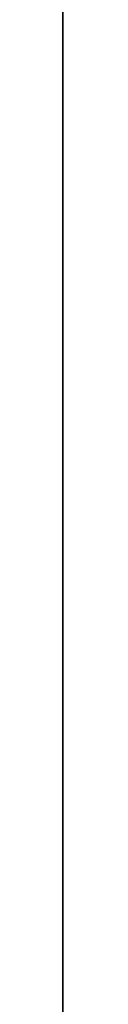
# Model space of a CAD drawing. Units: inches. Extents: x 2083 to 3317, y 1141 to 2115.
# Tile 33 of 256: x 2235.95977 to 2235.95984, y 1477.77958 to 1477.8005. Entities that reach past the tile are written whole.
import ezdxf

# ---------------------------------------------------------------- set-up
doc = ezdxf.new("R2010")
doc.units = ezdxf.units.IN
doc.layers.add('A-ANNO-DIMS', color=2, linetype='Continuous', lineweight=18)
doc.layers.add('A-WALL', color=7, linetype='Continuous', lineweight=35)
doc.layers.add('A-WALL-PATT', color=251, linetype='Continuous', lineweight=13, true_color=0x636466)
doc.styles.get("Standard").update_dxf_attribs({"font": 'arial.ttf'})
doc.dimstyles.new('ISO-25', dxfattribs={"dimtxt": 12, "dimasz": 12, "dimexe": 1.25, "dimexo": 0.625, "dimtad": 1, "dimlunit": 3, "dimtxsty": 'Standard', "dimcen": 2.5, "dimadec": 0, "dimazin": 0, "dimtfac": 1, "dimtmove": 0, "dimatfit": 3, "dimfxl": 1, "dimarcsym": 0})

# ---------------------------------------------------------------- blocks, each defined once
blk = doc.blocks.new('*D30')
at = {"layer": 'A-ANNO-DIMS', "color": 0, "lineweight": -2, "transparency": 16777216}
for p, q in [((2240.017856, 1445.273807), (2240.017856, 1448.045528)), ((2254.329327, 1445.273807), (2254.329327, 1448.045528)), ((2228.017856, 1446.795528), (2216.017856, 1446.795528)), ((2240.017856, 1446.795528), (2254.329327, 1446.795528)), ((2266.329327, 1446.795528), (2413.764866, 1446.795528))]:
    blk.add_line(p, q, dxfattribs=at)
at = {"layer": 'A-ANNO-DIMS', "color": 0, "transparency": 16777216}
for points in [[(2228.017856, 1448.795528), (2228.017856, 1444.795528), (2240.017856, 1446.795528)], [(2266.329327, 1448.795528), (2266.329327, 1444.795528), (2254.329327, 1446.795528)]]:
    blk.add_solid(points, dxfattribs=at)
at = {"layer": 'Defpoints', "color": 0, "transparency": 16777216}
for p in [(2254.329327, 1446.795528), (2240.017856, 1444.648807), (2254.329327, 1444.648807)]:
    blk.add_point(p, dxfattribs=at)
at = {"layer": 'A-ANNO-DIMS', "color": 0, "transparency": 16777216, "insert": (2346.047096, 1453.625167), "char_height": 12, "attachment_point": 5}
blk.add_mtext('WC 1\'-2 1/2" TYP.', dxfattribs=at)
blk = doc.blocks.new('*D31')
at = {"layer": 'A-ANNO-DIMS', "color": 0, "lineweight": -2, "transparency": 16777216}
for p, q in [((2237.871136, 1456.648807), (2237.871136, 1541.915179)), ((2239.392856, 1444.648807), (2236.621136, 1444.648807)), ((2237.871136, 1431.547542), (2237.871136, 1444.648807)), ((2239.392856, 1431.547542), (2236.621136, 1431.547542)), ((2237.871136, 1419.547542), (2237.871136, 1407.547542))]:
    blk.add_line(p, q, dxfattribs=at)
at = {"layer": 'A-ANNO-DIMS', "color": 0, "transparency": 16777216}
for points in [[(2235.871136, 1456.648807), (2239.871136, 1456.648807), (2237.871136, 1444.648807)], [(2235.871136, 1419.547542), (2239.871136, 1419.547542), (2237.871136, 1431.547542)]]:
    blk.add_solid(points, dxfattribs=at)
at = {"layer": 'Defpoints', "color": 0, "transparency": 16777216}
for p in [(2237.871136, 1444.648807), (2240.017856, 1444.648807), (2240.017856, 1431.547542)]:
    blk.add_point(p, dxfattribs=at)
at = {"layer": 'A-ANNO-DIMS', "color": 0, "transparency": 16777216, "insert": (2231.217486, 1505.281993), "char_height": 12, "attachment_point": 5, "rotation": 90}
blk.add_mtext('1\'-1" TYP.', dxfattribs=at)
blk = doc.blocks.new('*D45')
at = {"layer": 'A-ANNO-DIMS', "color": 0, "lineweight": -2, "transparency": 16777216}
for p, q in [((2235.959783, 1478.38636), (2235.959783, 1531.36136)), ((2418.959783, 1478.38636), (2418.959783, 1531.36136)), ((2247.959783, 1530.11136), (2406.959783, 1530.11136))]:
    blk.add_line(p, q, dxfattribs=at)
at = {"layer": 'A-ANNO-DIMS', "color": 0, "transparency": 16777216}
for points in [[(2247.959783, 1532.11136), (2247.959783, 1528.11136), (2235.959783, 1530.11136)], [(2406.959783, 1532.11136), (2406.959783, 1528.11136), (2418.959783, 1530.11136)]]:
    blk.add_solid(points, dxfattribs=at)
at = {"layer": 'Defpoints', "color": 0, "transparency": 16777216}
for p in [(2418.959783, 1530.11136), (2235.959783, 1477.76136), (2418.959783, 1477.76136)]:
    blk.add_point(p, dxfattribs=at)
at = {"layer": 'A-ANNO-DIMS', "color": 0, "transparency": 16777216, "insert": (2327.459783, 1536.867329), "char_height": 12, "attachment_point": 5}
blk.add_mtext('15\'-3"', dxfattribs=at)
blk = doc.blocks.new('*D62')
at = {"layer": 'A-ANNO-DIMS', "color": 0, "lineweight": -2, "transparency": 16777216}
for p, q in [((2235.959783, 1469.38636), (2235.959783, 1522.36136)), ((2379.959783, 1469.38636), (2379.959783, 1522.36136)), ((2247.959783, 1521.11136), (2367.959783, 1521.11136))]:
    blk.add_line(p, q, dxfattribs=at)
at = {"layer": 'A-ANNO-DIMS', "color": 0, "transparency": 16777216}
for points in [[(2247.959783, 1523.11136), (2247.959783, 1519.11136), (2235.959783, 1521.11136)], [(2367.959783, 1523.11136), (2367.959783, 1519.11136), (2379.959783, 1521.11136)]]:
    blk.add_solid(points, dxfattribs=at)
at = {"layer": 'Defpoints', "color": 0, "transparency": 16777216}
for p in [(2379.959783, 1521.11136), (2235.959783, 1468.76136), (2379.959783, 1468.76136)]:
    blk.add_point(p, dxfattribs=at)
at = {"layer": 'A-ANNO-DIMS', "color": 0, "transparency": 16777216, "insert": (2307.959783, 1527.863236), "char_height": 12, "attachment_point": 5}
blk.add_mtext('12\'-0"', dxfattribs=at)

msp = doc.modelspace()

# ---------------------------------------------------------------- hatches: boundary and pattern name
at = {"layer": 'A-WALL-PATT'}
h = msp.add_hatch(color=256, dxfattribs=at)
h.dxf.hatch_style = 1
h.paths.add_polyline_path([(3126.959783, 2020.76136), (2748.959783, 2020.76136), (2604.959783, 2020.76136), (2226.959783, 2020.76136), (2226.959783, 1702.76136), (2466.959783, 1702.76136), (2466.959783, 1582.76136), (2418.959783, 1582.76136), (2418.959783, 1477.76136), (2226.959783, 1477.76136), (2226.959783, 1263.26136), (2544.959783, 1263.26136), (2544.959783, 1411.76136), (2604.959783, 1411.76136), (2685.959783, 1411.76136), (2685.959783, 1420.76136), (2604.959783, 1420.76136), (2604.959783, 1573.76136), (2604.959783, 1702.76136), (2604.959783, 2011.76136), (2748.959783, 2011.76136), (2748.959783, 1702.76136), (2862.959783, 1702.76136), (2862.959783, 1621.76136), (2871.959783, 1621.76136), (2871.959783, 1702.76136), (2883.959783, 1702.76136), (2883.959783, 1706.939459, -0.026459), (2883.959783, 1711.76136), (2757.959783, 1711.76136), (2757.959783, 1807.76136), (2787.959783, 1807.76136), (2787.959783, 1812.26136), (2757.959783, 1812.26136), (2757.959783, 2011.76136), (2877.959783, 2011.76136), (2877.959783, 1812.26136), (2847.959783, 1812.26136), (2847.959783, 1807.76136), (2889.835742, 1807.76136), (2889.835742, 1812.26136), (2882.459783, 1812.26136), (2882.459783, 2011.76136), (3117.959783, 2011.76136), (3117.959783, 1812.26136), (2937.835742, 1812.26136), (2937.835742, 1807.76136), (2995.709783, 1807.76136), (2995.709783, 1796.117666), (3000.209783, 1796.117666), (3000.209783, 1807.76136), (3117.959783, 1807.76136), (3117.959783, 1711.76136), (3000.209783, 1711.76136), (3000.209783, 1760.117666), (2998.572705, 1760.117666, -0.020711), (2995.709783, 1760.117666), (2995.709783, 1711.76136), (2931.959783, 1711.76136), (2931.959783, 1702.76136), (3126.959783, 1702.76136)])
h.paths.add_polyline_path([(2471.459783, 2011.76136), (2471.459783, 1810.01136), (2462.716936, 1810.01136), (2462.716936, 1805.51136), (2505.959783, 1805.51136), (2505.959783, 1810.01136), (2475.959783, 1810.01136), (2475.959783, 2011.76136), (2595.959783, 2011.76136), (2595.959783, 1810.01136), (2565.959783, 1810.01136), (2565.959783, 1805.51136), (2595.959783, 1805.51136), (2595.959783, 1711.76136), (2235.959783, 1711.76136), (2235.959783, 1805.51136), (2353.709783, 1805.51136), (2353.709783, 1796.054162), (2358.209783, 1796.054162), (2358.209783, 1805.51136), (2414.716936, 1805.51136), (2414.716936, 1810.01136), (2235.959783, 1810.01136), (2235.959783, 2011.76136)], flags=16)
h.paths.add_polyline_path([(2270.204734, 1994.610008), (2270.204734, 1970.610008), (2246.204734, 1970.610008), (2246.204734, 1994.610008)], flags=0)
edge = h.paths.add_edge_path(flags=0)
edge.add_ellipse((2332.027391, 1899.798176), major_axis=(-3.042994, 3.042994), ratio=0.16825245, start_angle=-161.332166, end_angle=-156.307114, ccw=False)
edge.add_ellipse((2333.082037, 1898.74353), major_axis=(-1.054646, 1.054646), ratio=0.4535321, start_angle=-123.371019, end_angle=-94.159107)
edge = h.paths.add_edge_path(flags=0)
edge.add_ellipse((2332.027391, 1968.87629), major_axis=(3.042994, 3.042994), ratio=0.16825245, start_angle=18.667834, end_angle=23.692886)
edge.add_spline(control_points=[(2332.925596, 1970.691105), (2332.226768, 1970.3361), (2330.893709, 1969.658905), (2328.41308, 1970.932138), (2327.203934, 1967.748712), (2324.709596, 1969.955589), (2322.532822, 1967.012354), (2320.012846, 1971.295812), (2317.680308, 1968.157845), (2316.040526, 1967.102047), (2315.426904, 1966.809602)], knot_values=[0, 0, 0, 0, 2.267059, 4.324559, 6.685584, 8.878641, 11.121502, 14.300359, 17.755284, 19.732645, 19.732645, 19.732645, 19.732645], degree=3, periodic=0)
edge.add_ellipse((2332.027391, 1968.87629), major_axis=(3.042994, 3.042994), ratio=0.16825245, start_angle=18.667834, end_angle=23.692886, ccw=False)
edge.add_ellipse((2333.082037, 1969.930936), major_axis=(1.054646, 1.054646), ratio=0.4535321, start_angle=56.628981, end_angle=85.840893, ccw=False)
edge = h.paths.add_edge_path(flags=0)
edge.add_spline(control_points=[(2296.428287, 1967.987908), (2293.627804, 1965.336314), (2287.703624, 1959.727094), (2299.74386, 1949.995699), (2294.532591, 1935.668528), (2290.573228, 1920.603512), (2293.394124, 1909.973691), (2296.185407, 1904.966543)], knot_values=[0.099185, 0.099185, 0.099185, 0.099185, 0.345301, 0.619822, 0.982653, 1.386093, 1.810555, 1.810555, 1.810555, 1.810555], degree=3, periodic=0)
edge.add_spline(control_points=[(2296.185407, 1904.966543), (2297.383582, 1902.6193), (2298.000969, 1901.949312), (2298.55297, 1901.468155)], knot_values=[0.006246, 0.006246, 0.006246, 0.006246, 0.055476, 0.055476, 0.055476, 0.055476], degree=3, periodic=0)
edge.add_spline(control_points=[(2298.55297, 1901.468155), (2297.258612, 1900.923224), (2295.225294, 1900.232126), (2293.060229, 1900.614205), (2292.101423, 1900.788415), (2292.089578, 1900.790568)], knot_values=[0.312835, 0.312835, 0.312835, 0.312835, 0.40178, 0.474987, 0.475903, 0.475903, 0.475903, 0.475903], degree=3, periodic=0)
edge.add_arc((2292.793646, 1904.664109), 3.937008, 215.420897, 259.698179, ccw=False)
edge.add_spline(control_points=[(2289.585314, 1902.382304), (2289.476652, 1902.535087), (2289.36848, 1902.688035), (2289.260865, 1902.84117)], knot_values=[0.102872, 0.102872, 0.102872, 0.102872, 0.116896, 0.116896, 0.116896, 0.116896], degree=3, periodic=0)
edge.add_spline(control_points=[(2289.260865, 1902.84117), (2288.686604, 1902.550192), (2287.640048, 1902.019902), (2285.881337, 1901.873954), (2283.852972, 1901.504352), (2281.719987, 1899.710538), (2278.466991, 1899.492942), (2276.157136, 1901.883202), (2272.258953, 1899.804071), (2267.777605, 1901.843183), (2262.243882, 1900.184033), (2257.414927, 1901.782061), (2254.318374, 1900.72612), (2253.178285, 1900.337343)], knot_values=[0, 0, 0, 0, 1.907977, 3.477176, 5.261074, 7.972851, 11.680248, 13.717921, 16.939592, 22.789562, 27.502503, 33.595215, 37.145618, 37.145618, 37.145618, 37.145618], degree=3, periodic=0)
edge.add_line((2253.178285, 1900.337343), (2250.24424, 1902.84117))
edge.add_line((2250.24424, 1902.84117), (2250.24424, 1965.833296))
edge.add_line((2250.24424, 1965.833296), (2253.178285, 1968.337123))
edge.add_spline(control_points=[(2253.178285, 1968.337123), (2254.318374, 1967.948346), (2257.414927, 1966.892405), (2262.243882, 1968.490433), (2267.777605, 1966.831283), (2271.52673, 1968.537217), (2273.875914, 1967.828289), (2274.206701, 1967.727642)], knot_values=[0, 0, 0, 0, 0.09018, 0.244935, 0.364644, 0.513233, 0.537855, 0.537855, 0.537855, 0.537855], degree=3, periodic=0)
edge.add_arc((2274.352887, 1963.793349), 3.937008, 72.051134, 92.127949, ccw=False)
edge.add_arc((2281.296933, 1985.230003), 18.596298, 252.0511336, 288.5657217)
edge.add_arc((2292.316717, 1956.02888), 12.646081, 71.0267879, 113.7782184, ccw=False)
edge = h.paths.add_edge_path(flags=0)
edge.add_spline(control_points=[(2274.899415, 1951.856195), (2275.066156, 1951.616592), (2275.232687, 1951.376588), (2275.397987, 1951.135855)], knot_values=[1.409916, 1.409916, 1.409916, 1.409916, 1.43159, 1.43159, 1.43159, 1.43159], degree=3, periodic=0)
edge.add_spline(control_points=[(2275.397987, 1951.135855), (2275.792106, 1950.561885), (2276.179231, 1949.983774), (2276.545546, 1949.397103)], knot_values=[1.358238, 1.358238, 1.358238, 1.358238, 1.409916, 1.409916, 1.409916, 1.409916], degree=3, periodic=0)
edge.add_line((2276.545546, 1949.397103), (2277.437289, 1947.862185))
edge.add_spline(control_points=[(2277.437289, 1947.862185), (2276.303834, 1945.673115), (2274.639698, 1942.426882), (2274.631615, 1938.0939), (2272.799124, 1930.85155), (2274.356426, 1943.897046), (2275.947681, 1947.923356), (2276.545546, 1949.397103)], knot_values=[0.005632, 0.005632, 0.005632, 0.005632, 0.186014, 0.266002, 0.357087, 0.59639, 0.739732, 0.739732, 0.739732, 0.739732], degree=3, periodic=0)
edge.add_spline(control_points=[(2276.545546, 1949.397103), (2276.179231, 1949.983774), (2275.792106, 1950.561885), (2275.397987, 1951.135855)], knot_values=[1.358238, 1.358238, 1.358238, 1.358238, 1.409916, 1.409916, 1.409916, 1.409916], degree=3, periodic=0)
edge.add_spline(control_points=[(2275.397987, 1951.135855), (2274.9425, 1950.080452), (2274.20776, 1948.025272), (2273.934602, 1944.851477), (2272.468534, 1937.627489), (2273.466216, 1945.696466), (2274.700615, 1951.059472), (2274.899415, 1951.856195)], knot_values=[0.104364, 0.104364, 0.104364, 0.104364, 0.189636, 0.269624, 0.36071, 0.600013, 0.644622, 0.644622, 0.644622, 0.644622], degree=3, periodic=0)
h.paths.add_polyline_path([(2269.167514, 1963.127573, -0.357527), (2268.170633, 1960.97637, -0.092561), (2268.170633, 1939.436325, -0.357527), (2269.167514, 1937.285122, -0.357527), (2267.01631, 1938.282002, -0.164785), (2254.685581, 1938.282002, -0.357527), (2252.534378, 1937.285122, -0.357527), (2253.531259, 1939.436325, -0.092561), (2253.531259, 1960.97637, -0.357527), (2252.534378, 1963.127573, -0.357527), (2254.685581, 1962.130692, -0.164785), (2267.01631, 1962.130692, -0.357527)], flags=0)
h.paths.add_polyline_path([(2248.874068, 1967.8018), (2248.874068, 1957.02771), (2249.457783, 1957.02771), (2249.457783, 1911.646756), (2248.874068, 1911.646756), (2248.874068, 1900.872666), (2246.511863, 1900.872666, 0.197327), (2244.149658, 1902.456873), (2244.149658, 1966.217592, 0.197327), (2246.511863, 1967.8018)], flags=0)
h.paths.add_polyline_path([(2269.167514, 1931.389344, -0.357527), (2268.170633, 1929.238141, -0.092561), (2268.170633, 1907.698096, -0.357527), (2269.167514, 1905.546893, -0.357527), (2267.01631, 1906.543774, -0.164785), (2254.685581, 1906.543774, -0.357527), (2252.534378, 1905.546893, -0.357527), (2253.531259, 1907.698096, -0.092561), (2253.531259, 1929.238141, -0.357527), (2252.534378, 1931.389344, -0.357527), (2254.685581, 1930.392463, -0.164785), (2267.01631, 1930.392463, -0.357527)], flags=0)
edge = h.paths.add_edge_path(flags=0)
edge.add_spline(control_points=[(2276.196858, 1906.723702), (2276.168144, 1909.028928), (2276.114049, 1913.371852), (2270.598417, 1924.924978), (2273.905175, 1919.012779), (2275.921711, 1916.262063), (2275.47457, 1912.402149), (2277.257874, 1910.380621), (2276.696044, 1908.225036), (2276.646218, 1906.813023), (2276.617825, 1906.008407)], knot_values=[0, 0, 0, 0, 8.61026, 16.221274, 18.843057, 23.804898, 27.440828, 29.356102, 31.203478, 33.650687, 33.650687, 33.650687, 33.650687], degree=3, periodic=0)
edge.add_spline(control_points=[(2276.617825, 1906.008407), (2276.623313, 1905.624144), (2276.497738, 1904.628661), (2275.441779, 1903.854725), (2274.937314, 1903.08045), (2274.85908, 1902.84117)], knot_values=[0.156488, 0.156488, 0.156488, 0.156488, 0.184398, 0.231376, 0.250598, 0.250598, 0.250598, 0.250598], degree=3, periodic=0)
edge.add_line((2274.85908, 1902.84117), (2276.50598, 1902.84117))
edge.add_spline(control_points=[(2276.50598, 1902.84117), (2276.788308, 1903.08494), (2277.665071, 1904.125196), (2278.249538, 1904.340738), (2277.653872, 1908.527387), (2278.15567, 1906.227808), (2278.100464, 1905.285948), (2278.846675, 1904.069005), (2277.856785, 1903.414948), (2277.874191, 1902.99105), (2277.903562, 1902.84117)], knot_values=[0.059574, 0.059574, 0.059574, 0.059574, 0.080753, 0.103741, 0.16972, 0.176036, 0.207137, 0.240474, 0.262341, 0.27366, 0.27366, 0.27366, 0.27366], degree=3, periodic=0)
edge.add_line((2277.903562, 1902.84117), (2280.029825, 1902.84117))
edge.add_spline(control_points=[(2280.029825, 1902.84117), (2279.888221, 1903.088398), (2279.499257, 1903.981551), (2280.152284, 1905.939349), (2278.103615, 1909.657757), (2279.762395, 1907.185285), (2280.3279, 1904.874861), (2280.485109, 1903.48959), (2281.463269, 1903.249432), (2281.758343, 1902.936497), (2281.834036, 1902.84117)], knot_values=[0.013856, 0.013856, 0.013856, 0.013856, 0.034874, 0.088867, 0.107879, 0.126738, 0.158714, 0.193757, 0.217487, 0.226722, 0.226722, 0.226722, 0.226722], degree=3, periodic=0)
edge.add_spline(control_points=[(2281.834036, 1902.84117), (2281.787535, 1902.826703), (2281.647022, 1902.782988), (2281.395527, 1902.85949), (2281.088077, 1902.985242), (2280.720683, 1903.060902), (2280.333451, 1903.025726), (2280.124767, 1902.898879), (2280.029825, 1902.84117)], knot_values=[0, 0, 0, 0, 0.14413, 0.435517, 0.749276, 1.153046, 1.548371, 1.878348, 1.878348, 1.878348, 1.878348], degree=3, periodic=0)
edge.add_line((2280.029825, 1902.84117), (2277.903562, 1902.84117))
edge.add_spline(control_points=[(2277.903562, 1902.84117), (2277.892855, 1902.795855), (2277.865396, 1902.679637), (2277.607479, 1902.687483), (2277.27405, 1902.8007), (2276.837921, 1902.619775), (2276.583807, 1902.789261), (2276.50598, 1902.84117)], knot_values=[0, 0, 0, 0, 0.127189, 0.326199, 0.628009, 1.24357, 1.515331, 1.515331, 1.515331, 1.515331], degree=3, periodic=0)
edge.add_line((2276.50598, 1902.84117), (2274.85908, 1902.84117))
edge.add_spline(control_points=[(2274.85908, 1902.84117), (2274.814437, 1902.898587), (2274.72513, 1903.013446), (2274.493477, 1903.118968), (2274.244285, 1902.960539), (2273.937121, 1903.184942), (2273.614039, 1902.983143), (2273.408316, 1902.883045), (2273.322254, 1902.84117)], knot_values=[0, 0, 0, 0, 0.21843, 0.436957, 0.687977, 0.990379, 1.398396, 1.69185, 1.69185, 1.69185, 1.69185], degree=3, periodic=0)
edge.add_spline(control_points=[(2273.322254, 1902.84117), (2273.61674, 1903.445692), (2274.273998, 1904.538253), (2276.027239, 1904.573702), (2276.206963, 1906.583637), (2276.196858, 1906.723702)], knot_values=[0.012227, 0.012227, 0.012227, 0.012227, 0.059472, 0.106218, 0.134458, 0.134458, 0.134458, 0.134458], degree=3, periodic=0)
h.paths.add_polyline_path([(2270.776054, 1897.789828), (2270.776054, 1873.789828), (2246.776054, 1873.789828), (2246.776054, 1897.789828)], flags=0)
h.paths.add_polyline_path([(2353.709783, 1760.005059), (2353.709783, 1760.054162), (2358.209783, 1760.054162, -0.033729)], flags=0)
h.paths.add_polyline_path([(2321.819119, 1737.529186), (2341.995327, 1737.529186, -0.414214), (2343.203273, 1736.321241), (2343.203273, 1721.020596, -0.414214), (2341.995327, 1719.812651), (2321.819119, 1719.812651, -0.414214), (2320.611173, 1721.020596), (2320.611173, 1736.321241, -0.414214)], flags=0)
h.paths.add_polyline_path([(2324.23501, 1736.321241), (2339.579436, 1736.321241, -0.414214), (2341.995327, 1733.905349), (2341.995327, 1725.44973, -0.414214), (2339.579436, 1723.033839), (2333.680588, 1723.033839), (2333.845317, 1722.045467, -0.870646), (2335.425399, 1721.825893, -0.767327), (2333.922694, 1721.423245), (2331.291024, 1721.423245, -0.767327), (2329.788319, 1721.825893, -0.870646), (2331.368401, 1722.045467), (2331.53313, 1723.033839), (2324.23501, 1723.033839, -0.414214), (2321.819119, 1725.44973), (2321.819119, 1733.905349, -0.414214)], flags=0)
h.paths.add_polyline_path([(2570.483789, 1928.615444), (2589.683789, 1928.615444), (2590.168829, 1928.615444), (2590.168829, 1904.993397), (2570.483789, 1904.993397)], flags=0)
h.paths.add_polyline_path([(2574.447324, 1927.263822, -1), (2572.828836, 1927.263822, -1)], flags=0)
h.paths.add_polyline_path([(2573.089867, 1926.940877), (2573.925032, 1927.776042), (2574.147743, 1927.553332), (2573.312577, 1926.718166)], flags=0)
h.paths.add_polyline_path([(2578.779065, 1919.729618, -1), (2571.591663, 1919.729618, -1)], flags=0)
h.paths.add_polyline_path([(2578.385364, 1919.729618, -1), (2571.985364, 1919.729618, -1)], flags=0)
h.paths.add_polyline_path([(2331.595764, 1729.476216, -1), (2333.617954, 1729.476216, -1)], flags=0)
h.paths.add_polyline_path([(2578.034228, 1927.263822, -1), (2576.41574, 1927.263822, -1)], flags=0)
h.paths.add_polyline_path([(2576.688851, 1927.531089), (2576.911562, 1927.753799), (2577.746728, 1926.918634), (2577.524017, 1926.695923)], flags=0)
h.paths.add_polyline_path([(2578.139065, 1909.859539, -1), (2572.231663, 1909.859539, -1)], flags=0)
h.paths.add_polyline_path([(2577.745364, 1909.859539, -1), (2572.625364, 1909.859539, -1)], flags=0)
h.paths.add_polyline_path([(2583.797718, 1927.263822, -1), (2582.179229, 1927.263822, -1)], flags=0)
h.paths.add_polyline_path([(2582.718649, 1927.753799), (2583.553814, 1926.918634), (2583.331103, 1926.695923), (2582.495938, 1927.531089)], flags=0)
h.paths.add_polyline_path([(2582.495938, 1927.531089), (2582.718649, 1927.753799), (2583.553814, 1926.918634), (2583.331103, 1926.695923)], flags=0)
h.paths.add_polyline_path([(2587.739065, 1920.529618, -1), (2581.831663, 1920.529618, -1)], flags=0)
h.paths.add_polyline_path([(2587.345364, 1920.529618, -1), (2582.225364, 1920.529618, -1)], flags=0)
h.paths.add_polyline_path([(2587.384622, 1927.263822, -1), (2585.766133, 1927.263822, -1)], flags=0)
h.paths.add_polyline_path([(2586.081993, 1926.980247), (2586.917158, 1927.815412), (2587.139869, 1927.592702), (2586.304703, 1926.757536)], flags=0)
h.paths.add_polyline_path([(2588.379065, 1910.659539, -1), (2581.191663, 1910.659539, -1)], flags=0)
h.paths.add_polyline_path([(2587.985364, 1910.659539, -1), (2581.585364, 1910.659539, -1)], flags=0)
h.paths.add_polyline_path([(2417.167729, 1729.477895), (2437.343937, 1729.477895, -0.414214), (2438.551883, 1728.26995), (2438.551883, 1712.969306, -0.414214), (2437.343937, 1711.76136), (2417.167729, 1711.76136, -0.414214), (2415.959783, 1712.969306), (2415.959783, 1728.26995, -0.414214)], flags=0)
h.paths.add_polyline_path([(2419.58362, 1728.26995), (2434.928046, 1728.26995, -0.414214), (2437.343937, 1725.854059), (2437.343937, 1717.39844, -0.414214), (2434.928046, 1714.982548), (2429.029199, 1714.982548), (2429.193927, 1713.994176, -0.870646), (2430.774009, 1713.774603, -0.767327), (2429.271304, 1713.371954), (2426.639634, 1713.371954, -0.767327), (2425.136929, 1713.774603, -0.870646), (2426.717011, 1713.994176), (2426.88174, 1714.982548), (2419.58362, 1714.982548, -0.414214), (2417.167729, 1717.39844), (2417.167729, 1725.854059, -0.414214)], flags=0)
h.paths.add_polyline_path([(2419.58362, 1728.26995), (2434.928046, 1728.26995, -0.414214), (2437.343937, 1725.854059), (2437.343937, 1717.39844, -0.414214), (2434.928046, 1714.982548), (2429.029199, 1714.982548), (2428.358118, 1719.009034), (2427.552821, 1719.009034), (2426.88174, 1714.982548), (2419.58362, 1714.982548, -0.414214), (2417.167729, 1717.39844), (2417.167729, 1725.854059, -0.414214)], flags=0)
h.paths.add_polyline_path([(2426.944374, 1721.424925, -1), (2428.966564, 1721.424925, -1)], flags=0)
h.paths.add_polyline_path([(2475.959783, 1702.76136), (2595.959783, 1702.76136), (2595.959783, 1582.76136), (2475.959783, 1582.76136)], flags=16)
h.paths.add_polyline_path([(2427.959783, 1573.76136), (2595.959783, 1573.76136), (2595.959783, 1468.76136), (2595.959783, 1420.76136), (2384.459783, 1420.76136), (2384.459783, 1468.76136), (2427.959783, 1468.76136)], flags=16)
h.paths.add_polyline_path([(2379.959783, 1468.76136), (2379.959783, 1420.76136), (2235.959783, 1420.76136), (2235.959783, 1468.76136)], flags=16)
h.paths.add_polyline_path([(2317.815996, 1466.695767), (2337.992205, 1466.695767, -0.414214), (2339.20015, 1465.487821), (2339.20015, 1450.187177, -0.414214), (2337.992205, 1448.979232), (2317.815996, 1448.979232, -0.414214), (2316.608051, 1450.187177), (2316.608051, 1465.487821, -0.414214)], flags=0)
h.paths.add_polyline_path([(2320.231887, 1465.487821), (2335.576313, 1465.487821, -0.414214), (2337.992205, 1463.07193), (2337.992205, 1454.616311, -0.414214), (2335.576313, 1452.20042), (2329.677466, 1452.20042), (2329.842195, 1451.212047, -0.870646), (2331.422276, 1450.992474, -0.767327), (2329.919571, 1450.589826), (2327.287902, 1450.589826, -0.767327), (2325.785197, 1450.992474, -0.870646), (2327.365278, 1451.212047), (2327.530007, 1452.20042), (2320.231887, 1452.20042, -0.414214), (2317.815996, 1454.616311), (2317.815996, 1463.07193, -0.414214)], flags=0)
h.paths.add_polyline_path([(2320.231887, 1465.487821), (2335.576313, 1465.487821, -0.414214), (2337.992205, 1463.07193), (2337.992205, 1454.616311, -0.414214), (2335.576313, 1452.20042), (2329.677466, 1452.20042), (2329.006385, 1456.226905), (2328.201088, 1456.226905), (2327.530007, 1452.20042), (2320.231887, 1452.20042, -0.414214), (2317.815996, 1454.616311), (2317.815996, 1463.07193, -0.414214)], flags=0)
h.paths.add_polyline_path([(2327.592641, 1458.642796, -1), (2329.614832, 1458.642796, -1)], flags=0)
h.paths.add_polyline_path([(2244.411744, 1433.340453), (2241.920945, 1433.340453, -0.414214), (2240.017856, 1435.243542), (2240.017856, 1440.952808, -0.414211), (2241.920925, 1442.855897), (2244.411744, 1442.855897, -1.976472)], flags=0)
h.paths.add_polyline_path([(2245.356888, 1434.397536, -0.414214), (2245.356888, 1441.798814, -2.144098)], flags=0)
h.paths.add_polyline_path([(2535.959783, 1416.26136), (2535.959783, 1272.26136), (2235.959783, 1272.26136), (2235.959783, 1416.26136)], flags=16)
h.paths.add_polyline_path([(2260.119561, 1384.292841), (2260.119561, 1362.038649), (2237.865369, 1362.038649), (2237.865369, 1384.292841)], flags=0)
edge = h.paths.add_edge_path(flags=0)
edge.add_line((2318.251847, 1362.093298), (2318.145797, 1362.000973))
edge.add_ellipse((2317.445116, 1360.431044), major_axis=(2.82164, 2.82164), ratio=0.16825245, start_angle=18.667834, end_angle=20.948127, ccw=False)
edge.add_ellipse((2318.423045, 1361.408974), major_axis=(0.977929, 0.977929), ratio=0.4535321, start_angle=56.628981, end_angle=70.226201, ccw=False)
edge = h.paths.add_edge_path(flags=0)
edge.add_line((2319.10737, 1295.571078), (2319.015044, 1295.677128))
edge.add_ellipse((2317.445116, 1296.377809), major_axis=(-2.82164, 2.82164), ratio=0.16825245, start_angle=-161.332166, end_angle=-159.051873, ccw=False)
edge.add_ellipse((2318.423045, 1295.39988), major_axis=(-0.977929, 0.977929), ratio=0.4535321, start_angle=-123.371019, end_angle=-109.773799)
edge = h.paths.add_edge_path(flags=0)
edge.add_spline(control_points=[(2284.210349, 1301.170219), (2284.580688, 1300.444719), (2284.891189, 1299.892024), (2285.159553, 1299.461018)], knot_values=[0.039066, 0.039066, 0.039066, 0.039066, 0.055476, 0.055476, 0.055476, 0.055476], degree=3, periodic=0)
edge.add_line((2285.159553, 1299.461018), (2284.210349, 1301.170219))
edge = h.paths.add_edge_path(flags=0)
edge.add_line((2280.412458, 1297.298013), (2283.369991, 1297.036122))
edge.add_line((2283.369991, 1297.036122), (2286.40569, 1297.92631))
edge.add_spline(control_points=[(2286.40569, 1297.92631), (2285.305487, 1297.463119), (2284.344777, 1297.129151), (2283.369991, 1297.036122)], knot_values=[0.394369, 0.394369, 0.394369, 0.394369, 0.475903, 0.475903, 0.475903, 0.475903], degree=3, periodic=0)
edge.add_spline(control_points=[(2283.369991, 1297.036122), (2283.28139, 1297.027666), (2282.316289, 1296.957336), (2281.312502, 1297.134479), (2280.423441, 1297.296016), (2280.412458, 1297.298013)], knot_values=[0.312835, 0.312835, 0.312835, 0.312835, 0.320246, 0.393453, 0.394369, 0.394369, 0.394369, 0.394369], degree=3, periodic=0)
edge = h.paths.add_edge_path(flags=0)
edge.add_line((2284.435561, 1359.607285), (2280.446291, 1355.328047))
edge.add_line((2280.446291, 1355.328047), (2279.579987, 1351.017754))
edge.add_line((2279.579987, 1351.017754), (2282.412974, 1346.580433))
edge.add_spline(control_points=[(2282.412974, 1346.580433), (2283.153331, 1345.589236), (2284.252896, 1344.028897), (2284.801037, 1342.387167), (2284.935162, 1341.805544)], knot_values=[1.240098, 1.240098, 1.240098, 1.240098, 1.332892, 1.382712, 1.382712, 1.382712, 1.382712], degree=3, periodic=0)
edge.add_spline(control_points=[(2284.935162, 1341.805544), (2285.319108, 1340.1406), (2285.233029, 1338.409204), (2284.909938, 1336.654122)], knot_values=[1.097484, 1.097484, 1.097484, 1.097484, 1.240098, 1.240098, 1.240098, 1.240098], degree=3, periodic=0)
edge.add_spline(control_points=[(2284.909938, 1336.654122), (2284.586848, 1334.89904), (2284.026745, 1333.120272), (2283.462644, 1331.360585)], knot_values=[0.95487, 0.95487, 0.95487, 0.95487, 1.097484, 1.097484, 1.097484, 1.097484], degree=3, periodic=0)
edge.add_line((2283.462644, 1331.360585), (2281.890376, 1326.153357))
edge.add_line((2281.890376, 1326.153357), (2280.756259, 1321.056089))
edge.add_line((2280.756259, 1321.056089), (2280.299205, 1316.001977))
edge.add_line((2280.299205, 1316.001977), (2280.715933, 1310.950068))
edge.add_line((2280.715933, 1310.950068), (2282.028094, 1305.972137))
edge.add_line((2282.028094, 1305.972137), (2284.210349, 1301.170219))
edge.add_spline(control_points=[(2284.210349, 1301.170219), (2283.340731, 1302.730185), (2282.611904, 1304.336493), (2282.028094, 1305.972137)], knot_values=[0.099185, 0.099185, 0.099185, 0.099185, 0.241799, 0.241799, 0.241799, 0.241799], degree=3, periodic=0)
edge.add_spline(control_points=[(2282.028094, 1305.972137), (2281.444283, 1307.60778), (2281.005489, 1309.272759), (2280.715933, 1310.950068)], knot_values=[0.241799, 0.241799, 0.241799, 0.241799, 0.384413, 0.384413, 0.384413, 0.384413], degree=3, periodic=0)
edge.add_spline(control_points=[(2280.715933, 1310.950068), (2280.433241, 1312.587613), (2280.289386, 1314.276959), (2280.298894, 1315.962032), (2280.299205, 1316.001977)], knot_values=[0.384413, 0.384413, 0.384413, 0.384413, 0.523647, 0.527028, 0.527028, 0.527028, 0.527028], degree=3, periodic=0)
edge.add_spline(control_points=[(2280.299205, 1316.001977), (2280.312326, 1317.686955), (2280.477871, 1319.367926), (2280.756259, 1321.056089)], knot_values=[0.527028, 0.527028, 0.527028, 0.527028, 0.669642, 0.669642, 0.669642, 0.669642], degree=3, periodic=0)
edge.add_spline(control_points=[(2280.756259, 1321.056089), (2281.034648, 1322.744252), (2281.42588, 1324.439608), (2281.890376, 1326.153357)], knot_values=[0.669642, 0.669642, 0.669642, 0.669642, 0.812256, 0.812256, 0.812256, 0.812256], degree=3, periodic=0)
edge.add_spline(control_points=[(2281.890376, 1326.153357), (2282.264383, 1327.533251), (2282.78787, 1329.26181), (2283.352751, 1331.01778), (2283.462644, 1331.360585)], knot_values=[0.812256, 0.812256, 0.812256, 0.812256, 0.927087, 0.95487, 0.95487, 0.95487, 0.95487], degree=3, periodic=0)
edge.add_line((2283.462644, 1331.360585), (2284.909938, 1336.654122))
edge.add_line((2284.909938, 1336.654122), (2284.935162, 1341.805544))
edge.add_line((2284.935162, 1341.805544), (2282.412974, 1346.580433))
edge.add_spline(control_points=[(2282.412974, 1346.580433), (2281.275127, 1348.103792), (2280.078447, 1349.570318), (2279.579987, 1351.017754)], knot_values=[1.382712, 1.382712, 1.382712, 1.382712, 1.525326, 1.525326, 1.525326, 1.525326], degree=3, periodic=0)
edge.add_spline(control_points=[(2279.579987, 1351.017754), (2279.443282, 1351.414721), (2279.136312, 1352.856922), (2279.73519, 1354.290385), (2280.446291, 1355.328047)], knot_values=[1.525326, 1.525326, 1.525326, 1.525326, 1.564439, 1.667941, 1.667941, 1.667941, 1.667941], degree=3, periodic=0)
edge.add_spline(control_points=[(2280.446291, 1355.328047), (2281.426113, 1356.757835), (2282.930837, 1358.18256), (2284.435561, 1359.607285)], knot_values=[1.667941, 1.667941, 1.667941, 1.667941, 1.810555, 1.810555, 1.810555, 1.810555], degree=3, periodic=0)
edge.add_arc((2280.623075, 1348.518181), 11.72618, 71.0267879, 113.7782184)
edge.add_arc((2270.404892, 1375.595156), 17.243567, 252.0511336, 288.5657217, ccw=False)
edge.add_arc((2263.965969, 1355.717847), 3.650622, 72.051134, 92.127949)
edge.add_arc((2263.965969, 1355.717847), 3.650622, 92.127949, 177.98513)
edge.add_spline(control_points=[(2260.317604, 1355.846199), (2260.260417, 1354.220668), (2260.551278, 1350.186547), (2262.999344, 1346.766251), (2264.472741, 1344.649024)], knot_values=[1.43159, 1.43159, 1.43159, 1.43159, 1.564144, 1.770695, 1.770695, 1.770695, 1.770695], degree=3, periodic=0)
edge.add_line((2264.472741, 1344.649024), (2264.93559, 1343.98253))
edge.add_spline(control_points=[(2263.801044, 1340.248105), (2263.843238, 1340.514088), (2264.067244, 1341.756465), (2264.512693, 1343.002453), (2264.935047, 1343.981083)], knot_values=[0.53657, 0.53657, 0.53657, 0.53657, 0.559349, 0.644622, 0.644622, 0.644622, 0.644622], degree=3, periodic=0)
edge.add_spline(control_points=[(2264.935047, 1343.981083), (2265.117771, 1343.714975), (2265.298875, 1343.447906), (2265.476756, 1343.179365)], knot_values=[1.384077, 1.384077, 1.384077, 1.384077, 1.409916, 1.409916, 1.409916, 1.409916], degree=3, periodic=0)
edge.add_spline(control_points=[(2265.476756, 1343.179365), (2265.654637, 1342.910823), (2265.829296, 1342.64081), (2265.99913, 1342.368812)], knot_values=[1.358238, 1.358238, 1.358238, 1.358238, 1.384077, 1.384077, 1.384077, 1.384077], degree=3, periodic=0)
edge.add_line((2265.99913, 1342.368812), (2266.826006, 1340.945547))
edge.add_spline(control_points=[(2266.826006, 1340.945547), (2268.894401, 1337.089691), (2271.398173, 1325.843001), (2270.516164, 1310.568557), (2275.919376, 1301.860609), (2277.789511, 1299.19945)], knot_values=[0.116896, 0.116896, 0.116896, 0.116896, 0.472987, 1.050969, 1.313793, 1.313793, 1.313793, 1.313793], degree=3, periodic=0)
edge.add_spline(control_points=[(2277.789511, 1299.19945), (2277.839405, 1299.128452), (2277.889428, 1299.057498), (2277.939572, 1298.986584)], knot_values=[0.109884, 0.109884, 0.109884, 0.109884, 0.116896, 0.116896, 0.116896, 0.116896], degree=3, periodic=0)
edge.add_line((2277.939572, 1298.986584), (2277.788849, 1299.199114))
edge.add_spline(control_points=[(2277.788849, 1299.199114), (2277.256582, 1298.929414), (2276.28635, 1298.437902), (2275.039352, 1298.334419), (2274.38333, 1298.238895), (2274.215254, 1298.209338)], knot_values=[33.12187, 33.12187, 33.12187, 33.12187, 35.029056, 36.598255, 37.144827, 37.144827, 37.144827, 37.144827], degree=3, periodic=0)
edge.add_line((2274.215254, 1298.209338), (2273.073147, 1297.892961))
edge.add_spline(control_points=[(2273.073147, 1297.892961), (2272.322936, 1297.579784), (2271.039151, 1296.510508), (2269.248395, 1296.226062), (2268.4231, 1296.374654)], knot_values=[26.532584, 26.532584, 26.532584, 26.532584, 29.198919, 31.839101, 31.839101, 31.839101, 31.839101], degree=3, periodic=0)
edge.add_line((2268.4231, 1296.374654), (2263.878501, 1297.457534))
edge.add_spline(control_points=[(2263.878501, 1297.457534), (2263.556077, 1297.359435), (2261.860306, 1296.838694), (2260.23878, 1297.282407), (2258.933454, 1297.516461)], knot_values=[15.919551, 15.919551, 15.919551, 15.919551, 16.939592, 21.226067, 21.226067, 21.226067, 21.226067], degree=3, periodic=0)
edge.add_line((2258.933454, 1297.516461), (2254.055233, 1297.32901))
edge.add_spline(control_points=[(2254.055233, 1297.32901), (2253.755525, 1297.295815), (2252.113683, 1297.165174), (2250.461869, 1297.544221), (2249.129686, 1297.667882)], knot_values=[5.306517, 5.306517, 5.306517, 5.306517, 6.276435, 10.613034, 10.613034, 10.613034, 10.613034], degree=3, periodic=0)
edge.add_line((2249.129686, 1297.667882), (2244.33165, 1296.877756))
edge.add_line((2244.33165, 1296.877756), (2241.611033, 1299.19945))
edge.add_line((2241.611033, 1299.19945), (2241.611033, 1357.609404))
edge.add_line((2241.611033, 1357.609404), (2244.33165, 1359.931097))
edge.add_line((2244.33165, 1359.931097), (2252.728823, 1359.542692))
edge.add_spline(control_points=[(2252.728823, 1359.542692), (2252.870939, 1359.54644), (2253.30574, 1359.548172), (2253.739845, 1359.514274), (2254.031742, 1359.482426)], knot_values=[0.233291, 0.233291, 0.233291, 0.233291, 0.244935, 0.268927, 0.268927, 0.268927, 0.268927], degree=3, periodic=0)
edge.add_line((2254.031742, 1359.482426), (2259.58719, 1359.41639))
edge.add_spline(control_points=[(2259.58719, 1359.41639), (2260.677068, 1359.628503), (2262.073197, 1359.897003), (2263.523692, 1359.459278), (2263.830417, 1359.365952)], knot_values=[0.422516, 0.422516, 0.422516, 0.422516, 0.513233, 0.537855, 0.537855, 0.537855, 0.537855], degree=3, periodic=0)
edge.add_arc((2263.965969, 1355.717847), 3.650622, 72.051134, 92.127949, ccw=False)
edge.add_arc((2270.404892, 1375.595156), 17.243567, 252.0511336, 288.5657217)
edge.add_arc((2280.623075, 1348.518181), 11.72618, 71.0267879, 113.7782184, ccw=False)
h.paths.add_polyline_path([(2240.34053, 1359.434715), (2240.34053, 1349.444353), (2240.881785, 1349.444353), (2240.881785, 1307.3645), (2240.34053, 1307.3645), (2240.34053, 1297.374138), (2238.150157, 1297.374138, 0.197327), (2235.959783, 1298.843108), (2235.959783, 1357.965746, 0.197327), (2238.150157, 1359.434715)], flags=0)
h.paths.add_polyline_path([(2259.15779, 1355.1005, -0.357527), (2258.233425, 1353.10578, -0.092561), (2258.233425, 1333.132601, -0.357527), (2259.15779, 1331.13788, -0.357527), (2257.16307, 1332.062246, -0.164785), (2245.729302, 1332.062246, -0.357527), (2243.734582, 1331.13788, -0.357527), (2244.658947, 1333.132601, -0.092561), (2244.658947, 1353.10578, -0.357527), (2243.734582, 1355.1005, -0.357527), (2245.729302, 1354.176135, -0.164785), (2257.16307, 1354.176135, -0.357527)], flags=0)
edge = h.paths.add_edge_path(flags=0)
edge.add_line((2265.99913, 1342.368812), (2266.826006, 1340.945547))
edge.add_line((2266.826006, 1340.945547), (2265.307557, 1337.814066))
edge.add_line((2265.307557, 1337.814066), (2264.358232, 1334.652939))
edge.add_line((2264.358232, 1334.652939), (2264.262012, 1333.799705))
edge.add_spline(control_points=[(2264.262012, 1333.799705), (2264.208357, 1333.187055), (2264.16206, 1332.365525), (2264.007144, 1331.413933), (2263.969049, 1331.201834)], knot_values=[0.464444, 0.464444, 0.464444, 0.464444, 0.516691, 0.531608, 0.531608, 0.531608, 0.531608], degree=3, periodic=0)
edge.add_spline(control_points=[(2263.969049, 1331.201834), (2263.774535, 1330.118873), (2263.42437, 1328.790839), (2263.25742, 1328.530652), (2263.234028, 1328.514612)], knot_values=[0.372682, 0.372682, 0.372682, 0.372682, 0.44885, 0.464444, 0.464444, 0.464444, 0.464444], degree=3, periodic=0)
edge.add_spline(control_points=[(2263.234028, 1328.514612), (2263.096382, 1328.420227), (2263.13117, 1329.301477), (2263.274953, 1330.615749)], knot_values=[0.280919, 0.280919, 0.280919, 0.280919, 0.372682, 0.372682, 0.372682, 0.372682], degree=3, periodic=0)
edge.add_spline(control_points=[(2263.274953, 1330.615749), (2263.418736, 1331.930022), (2263.671515, 1333.677318), (2263.969852, 1335.315027)], knot_values=[0.189157, 0.189157, 0.189157, 0.189157, 0.280919, 0.280919, 0.280919, 0.280919], degree=3, periodic=0)
edge.add_spline(control_points=[(2263.969852, 1335.315027), (2264.100496, 1336.032192), (2264.418783, 1337.621911), (2264.754848, 1338.86443), (2264.947419, 1339.491124)], knot_values=[0.097394, 0.097394, 0.097394, 0.097394, 0.137578, 0.189157, 0.189157, 0.189157, 0.189157], degree=3, periodic=0)
edge.add_spline(control_points=[(2264.947419, 1339.491124), (2265.290017, 1340.606055), (2265.644238, 1341.493996), (2265.99913, 1342.368812)], knot_values=[0.005632, 0.005632, 0.005632, 0.005632, 0.097394, 0.097394, 0.097394, 0.097394], degree=3, periodic=0)
h.paths.add_polyline_path([(2259.15779, 1325.670973, -0.357527), (2258.233425, 1323.676253, -0.092561), (2258.233425, 1303.703073, -0.357527), (2259.15779, 1301.708353, -0.357527), (2257.16307, 1302.632719, -0.164785), (2245.729302, 1302.632719, -0.357527), (2243.734582, 1301.708353, -0.357527), (2244.658947, 1303.703073, -0.092561), (2244.658947, 1323.676253, -0.357527), (2243.734582, 1325.670973, -0.357527), (2245.729302, 1324.746608, -0.164785), (2257.16307, 1324.746608, -0.357527)], flags=0)
edge = h.paths.add_edge_path(flags=0)
edge.add_spline(control_points=[(2261.708938, 1317.311421), (2261.679482, 1317.41758), (2261.761858, 1317.388535), (2262.490736, 1316.089873), (2262.962185, 1315.300897)], knot_values=[14.955861, 14.955861, 14.955861, 14.955861, 16.221274, 18.694826, 18.694826, 18.694826, 18.694826], degree=3, periodic=0)
edge.add_spline(control_points=[(2262.962185, 1315.300897), (2262.990437, 1315.253617), (2263.702096, 1314.067376), (2264.348983, 1313.127153), (2264.730054, 1312.164154)], knot_values=[18.694826, 18.694826, 18.694826, 18.694826, 18.843057, 22.433791, 22.433791, 22.433791, 22.433791], degree=3, periodic=0)
edge.add_spline(control_points=[(2264.730054, 1312.164154), (2264.875565, 1311.796437), (2265.176873, 1310.769807), (2265.143069, 1309.559262), (2265.247736, 1308.824193)], knot_values=[22.433791, 22.433791, 22.433791, 22.433791, 23.804898, 26.172756, 26.172756, 26.172756, 26.172756], degree=3, periodic=0)
edge.add_line((2265.247736, 1308.824193), (2265.850774, 1307.171888))
edge.add_spline(control_points=[(2265.850774, 1307.171888), (2266.065025, 1306.821678), (2266.384387, 1306.332246), (2266.4244, 1305.780549), (2266.420369, 1305.611216)], knot_values=[28.062562, 28.062562, 28.062562, 28.062562, 29.356102, 29.911721, 29.911721, 29.911721, 29.911721], degree=3, periodic=0)
edge.add_spline(control_points=[(2266.420369, 1305.611216), (2266.416116, 1305.43259), (2266.393999, 1305.249998), (2266.364777, 1305.065857)], knot_values=[29.911721, 29.911721, 29.911721, 29.911721, 30.497837, 30.497837, 30.497837, 30.497837], degree=3, periodic=0)
edge.add_line((2266.364777, 1305.065857), (2266.066151, 1302.136295))
edge.add_spline(control_points=[(2266.066151, 1302.136295), (2266.07124, 1301.779984), (2265.998076, 1301.199985), (2265.663266, 1300.758961), (2265.508908, 1300.585882)], knot_values=[0.156488, 0.156488, 0.156488, 0.156488, 0.184398, 0.203543, 0.203543, 0.203543, 0.203543], degree=3, periodic=0)
edge.add_line((2265.508908, 1300.585882), (2264.435341, 1299.19945))
edge.add_line((2264.435341, 1299.19945), (2265.962442, 1299.19945))
edge.add_line((2265.962442, 1299.19945), (2267.33599, 1301.175276))
edge.add_line((2267.33599, 1301.175276), (2267.311667, 1301.986237))
edge.add_spline(control_points=[(2267.311667, 1301.986237), (2267.261111, 1302.862396), (2267.160212, 1303.737132), (2267.271486, 1303.325896)], knot_values=[0.126229, 0.126229, 0.126229, 0.126229, 0.166617, 0.166617, 0.166617, 0.166617], degree=3, periodic=0)
edge.add_spline(control_points=[(2267.271486, 1303.325896), (2267.280035, 1303.294305), (2267.309785, 1303.175366), (2267.37345, 1302.883608), (2267.406123, 1302.682829), (2267.417926, 1302.601025)], knot_values=[0.166617, 0.166617, 0.166617, 0.166617, 0.16972, 0.176036, 0.180765, 0.180765, 0.180765, 0.180765], degree=3, periodic=0)
edge.add_spline(control_points=[(2267.743891, 1300.987505), (2267.687583, 1301.150943), (2267.48052, 1301.656664), (2267.483751, 1302.144788), (2267.417926, 1302.601025)], knot_values=[0.180765, 0.180765, 0.180765, 0.180765, 0.193767, 0.220139, 0.220139, 0.220139, 0.220139], degree=3, periodic=0)
edge.add_line((2267.417926, 1302.601025), (2267.743891, 1300.987505))
edge.add_spline(control_points=[(2267.743891, 1300.987505), (2267.831961, 1300.731878), (2267.932021, 1300.309904), (2267.554841, 1299.974518), (2267.429366, 1299.829207)], knot_values=[0.220139, 0.220139, 0.220139, 0.220139, 0.240474, 0.25489, 0.25489, 0.25489, 0.25489], degree=3, periodic=0)
edge.add_line((2267.429366, 1299.829207), (2267.258361, 1299.19945))
edge.add_line((2267.258361, 1299.19945), (2269.229956, 1299.19945))
edge.add_spline(control_points=[(2269.229956, 1299.19945), (2269.098653, 1299.428694), (2268.842774, 1300.016251), (2269.011575, 1300.915923), (2268.946796, 1301.66074)], knot_values=[0.013856, 0.013856, 0.013856, 0.013856, 0.034874, 0.067073, 0.067073, 0.067073, 0.067073], degree=3, periodic=0)
edge.add_line((2268.946796, 1301.66074), (2268.431582, 1303.603109))
edge.add_spline(control_points=[(2268.431582, 1303.603109), (2268.175596, 1304.192375), (2267.596214, 1305.251298), (2268.040698, 1304.62321), (2268.251394, 1304.282421)], knot_values=[0.090155, 0.090155, 0.090155, 0.090155, 0.107879, 0.120289, 0.120289, 0.120289, 0.120289], degree=3, periodic=0)
edge.add_spline(control_points=[(2268.251394, 1304.282421), (2268.360882, 1304.105329), (2269.057753, 1302.917983), (2269.382691, 1301.590419), (2269.521405, 1300.775931), (2269.57522, 1300.555784)], knot_values=[0.120289, 0.120289, 0.120289, 0.120289, 0.126738, 0.158714, 0.173506, 0.173506, 0.173506, 0.173506], degree=3, periodic=0)
edge.add_line((2269.57522, 1300.555784), (2270.685798, 1299.421258))
edge.add_spline(control_points=[(2270.685798, 1299.421258), (2270.767221, 1299.357251), (2270.837852, 1299.281401), (2270.902925, 1299.19945)], knot_values=[0.21816, 0.21816, 0.21816, 0.21816, 0.226722, 0.226722, 0.226722, 0.226722], degree=3, periodic=0)
edge.add_line((2270.937201, 1299.192913), (2270.902925, 1299.19945))
edge.add_spline(control_points=[(2270.902925, 1299.19945), (2270.859806, 1299.186035), (2270.729515, 1299.1455), (2270.496314, 1299.216437), (2270.271661, 1299.308323), (2270.121017, 1299.347961), (2270.063339, 1299.359557)], knot_values=[0.939174, 0.939174, 0.939174, 0.939174, 1.083304, 1.374691, 1.68845, 1.878348, 1.878348, 1.878348, 1.878348], degree=3, periodic=0)
edge.add_line((2270.063339, 1299.359557), (2269.229956, 1299.19945))
edge.add_line((2269.229956, 1299.19945), (2267.258361, 1299.19945))
edge.add_spline(control_points=[(2267.258361, 1299.19945), (2267.248433, 1299.157431), (2267.222971, 1299.049667), (2266.983816, 1299.056942), (2266.80921, 1299.11623), (2266.676905, 1299.109091), (2266.636531, 1299.104815)], knot_values=[0.757665, 0.757665, 0.757665, 0.757665, 0.884854, 1.083864, 1.385675, 1.515331, 1.515331, 1.515331, 1.515331], degree=3, periodic=0)
edge.add_spline(control_points=[(2266.636531, 1299.104815), (2266.485225, 1299.088788), (2266.235807, 1299.017123), (2266.034608, 1299.151317), (2265.962442, 1299.19945)], knot_values=[0, 0, 0, 0, 0.485905, 0.757665, 0.757665, 0.757665, 0.757665], degree=3, periodic=0)
edge.add_line((2265.962442, 1299.19945), (2264.435341, 1299.19945))
edge.add_line((2264.435341, 1299.19945), (2263.858444, 1299.367118))
edge.add_spline(control_points=[(2263.858444, 1299.367118), (2263.818943, 1299.370905), (2263.779528, 1299.385721), (2263.740131, 1299.401504)], knot_values=[0.845925, 0.845925, 0.845925, 0.845925, 0.978627, 0.978627, 0.978627, 0.978627], degree=3, periodic=0)
edge.add_line((2263.721786, 1299.396425), (2263.010306, 1299.19945))
edge.add_spline(control_points=[(2263.010306, 1299.19945), (2263.245794, 1299.682859), (2263.506032, 1300.128107), (2263.873494, 1300.408028)], knot_values=[0.012227, 0.012227, 0.012227, 0.012227, 0.052971, 0.052971, 0.052971, 0.052971], degree=3, periodic=0)
edge.add_spline(control_points=[(2263.873494, 1300.408028), (2263.932131, 1300.452695), (2264.084243, 1300.552979), (2264.255189, 1300.624223), (2264.359686, 1300.664747)], knot_values=[0.052971, 0.052971, 0.052971, 0.052971, 0.059472, 0.069086, 0.069086, 0.069086, 0.069086], degree=3, periodic=0)
edge.add_line((2264.359686, 1300.664747), (2265.1419, 1301.077774))
edge.add_line((2265.1419, 1301.077774), (2265.675806, 1302.799558))
edge.add_line((2265.675806, 1302.799558), (2265.5407, 1305.704066))
edge.add_line((2265.5407, 1305.704066), (2264.803073, 1309.327724))
edge.add_line((2264.803073, 1309.327724), (2263.040535, 1314.091791))
edge.add_spline(control_points=[(2263.040535, 1314.091791), (2262.383572, 1315.671438), (2261.795972, 1316.997749), (2261.708938, 1317.311421)], knot_values=[11.216896, 11.216896, 11.216896, 11.216896, 14.955861, 14.955861, 14.955861, 14.955861], degree=3, periodic=0)
h.paths.add_polyline_path([(2871.959783, 1416.26136), (2895.910047, 1416.26136), (2895.910047, 1420.76136), (2871.959783, 1420.76136), (2871.959783, 1501.76136), (2862.959783, 1501.76136), (2862.959783, 1420.76136), (2805.959783, 1420.76136), (2805.959783, 1411.76136), (2862.959783, 1411.76136), (2862.959783, 1263.26136), (3126.959783, 1263.26136), (3126.959783, 1411.76136), (3126.959783, 1486.76136), (2943.959783, 1486.76136), (2943.959783, 1477.76136), (2967.860311, 1477.76136), (2967.860311, 1420.76136), (2943.910047, 1420.76136), (2943.910047, 1416.26136), (3117.959783, 1416.26136), (3117.959783, 1420.76136), (2972.360311, 1420.76136), (2972.360311, 1477.76136), (3117.959783, 1477.76136), (3117.959783, 1420.76136), (3117.959783, 1272.26136), (2871.959783, 1272.26136)], flags=0)
h.paths.add_polyline_path([(2457.125626, 1485.942505), (2527.602651, 1485.942505), (2527.602651, 1537.635702), (2457.125626, 1537.635702)], flags=8)
h.paths.add_polyline_path([(2481.005058, 1609.981804), (2590.765818, 1609.981804), (2590.765818, 1682.003362), (2481.005058, 1682.003362)], flags=8)
h.paths.add_polyline_path([(2483.085022, 1729.126784), (2553.562048, 1729.126784), (2553.562048, 1780.81998), (2483.085022, 1780.81998)], flags=8)

# ---------------------------------------------------------------- linework, layer by layer
at = {"layer": 'A-WALL'}
msp.add_line((2235.959783, 1702.76136), (2235.959783, 1477.76136), dxfattribs=at)
msp.add_line((2235.959783, 1702.76136), (2235.959783, 1477.76136), dxfattribs=at)

# ---------------------------------------------------------------- dimensions: what is measured, and where the dimension line sits
at = {"layer": 'A-ANNO-DIMS'}
for base, p1, p2, picture, middle in [((2418.959783, 1530.11136), (2235.959783, 1477.76136), (2418.959783, 1477.76136), '*D45', (2327.459783, 1536.867329)), ((2379.959783, 1521.11136), (2235.959783, 1468.76136), (2379.959783, 1468.76136), '*D62', (2307.959783, 1527.863236))]:
    dim = msp.add_linear_dim(base=base, p1=p1, p2=p2, dimstyle='ISO-25', override={"dimdec": 1, "dimlfac": 1, "dimrnd": 0, "dimzin": 1, "dimdsep": 46, "dimlunit": 4, "dimfrac": 2}, dxfattribs=at)
    dim.commit()
    dim.dimension.update_dxf_attribs({"geometry": picture, "text_midpoint": middle})
dim = msp.add_linear_dim(base=(2237.871136, 1444.648807), p1=(2240.017856, 1431.547542), p2=(2240.017856, 1444.648807), angle=90, text='<> TYP.', dimstyle='ISO-25', override={"dimdec": 1, "dimlfac": 1, "dimrnd": 0, "dimzin": 1, "dimdsep": 46, "dimlunit": 4, "dimfrac": 2}, dxfattribs=at)
dim.commit()
dim.dimension.update_dxf_attribs({"geometry": '*D31', "text_midpoint": (2231.217486, 1505.281993)})
dim = msp.add_linear_dim(base=(2254.329327, 1446.795528), p1=(2240.017856, 1444.648807), p2=(2254.329327, 1444.648807), text='WC <> TYP.', dimstyle='ISO-25', override={"dimdec": 1, "dimlfac": 1, "dimrnd": 0, "dimzin": 1, "dimdsep": 46, "dimlunit": 4, "dimfrac": 2}, dxfattribs=at)
dim.commit()
dim.dimension.update_dxf_attribs({"geometry": '*D30', "text_midpoint": (2346.047096, 1453.625167)})

doc.saveas('drawing.dxf')
